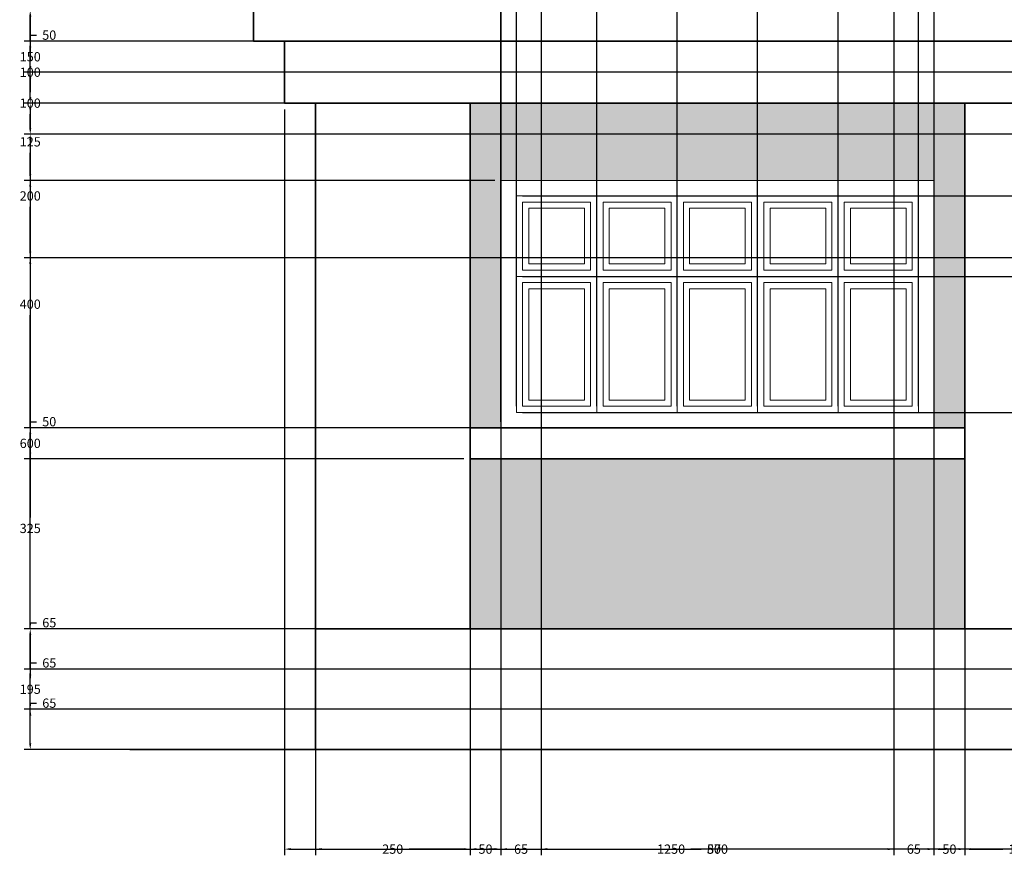
# Model space of a CAD drawing. Units: millimetres. Extents: x 937 to 4561, y 2711 to 5748.
# Tile 1 of 8: x 951 to 2543, y 2711 to 4062. Entities that reach past the tile are written whole.
import ezdxf

# ---------------------------------------------------------------- set-up
doc = ezdxf.new("R2010")
doc.units = ezdxf.units.MM
doc.header["$MEASUREMENT"] = 0
for name, color, linetype, lineweight in [('A-ANNO-DIMS', 2, 'Continuous', 18), ('A-ELEV', 7, 'Continuous', 35), ('A-GLAZ', 4, 'Continuous', 18), ('A-WALL-PATT', 8, 'Continuous', 13)]:
    doc.layers.add(name, color=color, linetype=linetype, lineweight=lineweight)
doc.styles.get("Standard").update_dxf_attribs({"font": 'arial.ttf'})
doc.dimstyles.get("Standard").update_dxf_attribs({"dimtxt": 15, "dimasz": 10, "dimexe": 10, "dimexo": 10, "dimgap": 10, "dimtad": 0, "dimtih": 1, "dimtoh": 1, "dimdec": 0, "dimzin": 0, "dimdsep": 46, "dimtxsty": 'Standard', "dimcen": 5, "dimadec": 0, "dimazin": 0, "dimtfac": 1, "dimtdec": 0, "dimtofl": 0, "dimtmove": 0, "dimatfit": 3, "dimfxl": 1, "dimtolj": 1, "dimtzin": 0, "dimarcsym": 0})

# ---------------------------------------------------------------- blocks, each defined once
blk = doc.blocks.new('*D4')
at = {"layer": 'A-ANNO-DIMS', "color": 0, "lineweight": -2, "transparency": 16777216}
for p, q in [((1429.5, 3066.9), (1429.5, 2710.9)), ((1679.5, 3066.9), (1679.5, 2710.9)), ((1439.5, 2720.9), (1527.8, 2720.9)), ((1669.5, 2720.9), (1581.2, 2720.9))]:
    blk.add_line(p, q, dxfattribs=at)
at = {"layer": 'A-ANNO-DIMS', "color": 0, "transparency": 16777216}
for points in [[(1439.5, 2722.6), (1439.5, 2719.2), (1429.5, 2720.9)], [(1669.5, 2722.6), (1669.5, 2719.2), (1679.5, 2720.9)]]:
    blk.add_solid(points, dxfattribs=at)
at = {"layer": 'Defpoints', "color": 0, "transparency": 16777216}
for p in [(1429.5, 3076.9), (1679.5, 3076.9), (1679.5, 2720.9)]:
    blk.add_point(p, dxfattribs=at)
at = {"layer": 'A-ANNO-DIMS', "color": 0, "transparency": 16777216, "insert": (1554.5, 2720.9), "char_height": 15, "attachment_point": 5}
blk.add_mtext('\\A1;250', dxfattribs=at)
blk = doc.blocks.new('*D5')
at = {"layer": 'A-ANNO-DIMS', "color": 0, "lineweight": -2, "transparency": 16777216}
for p, q in [((1679.5, 3066.9), (1679.5, 2710.9)), ((2479.5, 3066.9), (2479.5, 2710.9)), ((1689.5, 2720.9), (2052.9, 2720.9)), ((2469.5, 2720.9), (2106, 2720.9))]:
    blk.add_line(p, q, dxfattribs=at)
at = {"layer": 'A-ANNO-DIMS', "color": 0, "transparency": 16777216}
for points in [[(1689.5, 2722.6), (1689.5, 2719.2), (1679.5, 2720.9)], [(2469.5, 2722.6), (2469.5, 2719.2), (2479.5, 2720.9)]]:
    blk.add_solid(points, dxfattribs=at)
at = {"layer": 'Defpoints', "color": 0, "transparency": 16777216}
for p in [(1679.5, 3076.9), (2479.5, 3076.9), (2479.5, 2720.9)]:
    blk.add_point(p, dxfattribs=at)
at = {"layer": 'A-ANNO-DIMS', "color": 0, "transparency": 16777216, "insert": (2079.5, 2720.9), "char_height": 15, "attachment_point": 5}
blk.add_mtext('\\A1;800', dxfattribs=at)
blk = doc.blocks.new('*D6')
at = {"layer": 'A-ANNO-DIMS', "color": 0, "lineweight": -2, "transparency": 16777216}
for p, q in [((2479.5, 3066.9), (2479.5, 2710.9)), ((2654.5, 3066.9), (2654.5, 2710.9)), ((2489.5, 2720.9), (2541.1, 2720.9)), ((2644.5, 2720.9), (2592.9, 2720.9))]:
    blk.add_line(p, q, dxfattribs=at)
at = {"layer": 'A-ANNO-DIMS', "color": 0, "transparency": 16777216}
for points in [[(2489.5, 2722.6), (2489.5, 2719.2), (2479.5, 2720.9)], [(2644.5, 2722.6), (2644.5, 2719.2), (2654.5, 2720.9)]]:
    blk.add_solid(points, dxfattribs=at)
at = {"layer": 'Defpoints', "color": 0, "transparency": 16777216}
for p in [(2479.5, 3076.9), (2654.5, 3076.9), (2654.5, 2720.9)]:
    blk.add_point(p, dxfattribs=at)
at = {"layer": 'A-ANNO-DIMS', "color": 0, "transparency": 16777216, "insert": (2567, 2720.9), "char_height": 15, "attachment_point": 5}
blk.add_mtext('\\A1;175', dxfattribs=at)
blk = doc.blocks.new('*D27')
at = {"layer": 'A-ANNO-DIMS', "color": 0, "lineweight": -2, "transparency": 16777216}
for p, q in [((1729.5, 4391.9), (1729.5, 2710.9)), ((1794.5, 4391.9), (1794.5, 2710.9)), ((1719.5, 2720.9), (1709.5, 2720.9)), ((1804.5, 2720.9), (1814.5, 2720.9))]:
    blk.add_line(p, q, dxfattribs=at)
at = {"layer": 'A-ANNO-DIMS', "color": 0, "transparency": 16777216}
for points in [[(1719.5, 2722.6), (1719.5, 2719.2), (1729.5, 2720.9)], [(1804.5, 2722.6), (1804.5, 2719.2), (1794.5, 2720.9)]]:
    blk.add_solid(points, dxfattribs=at)
at = {"layer": 'Defpoints', "color": 0, "transparency": 16777216}
for p in [(1729.5, 4401.9), (1794.5, 4401.9), (1794.5, 2720.9)]:
    blk.add_point(p, dxfattribs=at)
at = {"layer": 'A-ANNO-DIMS', "color": 0, "transparency": 16777216, "insert": (1762, 2720.9), "char_height": 15, "attachment_point": 5}
blk.add_mtext('\\A1;65', dxfattribs=at)
blk = doc.blocks.new('*D28')
at = {"layer": 'A-ANNO-DIMS', "color": 0, "lineweight": -2, "transparency": 16777216}
for p, q in [((1794.5, 4391.9), (1794.5, 2710.9)), ((2364.5, 4391.9), (2364.5, 2710.9)), ((1804.5, 2720.9), (2052.9, 2720.9)), ((2354.5, 2720.9), (2106, 2720.9))]:
    blk.add_line(p, q, dxfattribs=at)
at = {"layer": 'A-ANNO-DIMS', "color": 0, "transparency": 16777216}
for points in [[(1804.5, 2722.6), (1804.5, 2719.2), (1794.5, 2720.9)], [(2354.5, 2722.6), (2354.5, 2719.2), (2364.5, 2720.9)]]:
    blk.add_solid(points, dxfattribs=at)
at = {"layer": 'Defpoints', "color": 0, "transparency": 16777216}
for p in [(1794.5, 4401.9), (2364.5, 4401.9), (2364.5, 2720.9)]:
    blk.add_point(p, dxfattribs=at)
at = {"layer": 'A-ANNO-DIMS', "color": 0, "transparency": 16777216, "insert": (2079.5, 2720.9), "char_height": 15, "attachment_point": 5}
blk.add_mtext('\\A1;570', dxfattribs=at)
blk = doc.blocks.new('*D29')
at = {"layer": 'A-ANNO-DIMS', "color": 0, "lineweight": -2, "transparency": 16777216}
for p, q in [((2364.5, 4391.9), (2364.5, 2710.9)), ((2429.5, 4391.9), (2429.5, 2710.9)), ((2354.5, 2720.9), (2344.5, 2720.9)), ((2439.5, 2720.9), (2449.5, 2720.9))]:
    blk.add_line(p, q, dxfattribs=at)
at = {"layer": 'A-ANNO-DIMS', "color": 0, "transparency": 16777216}
for points in [[(2354.5, 2722.6), (2354.5, 2719.2), (2364.5, 2720.9)], [(2439.5, 2722.6), (2439.5, 2719.2), (2429.5, 2720.9)]]:
    blk.add_solid(points, dxfattribs=at)
at = {"layer": 'Defpoints', "color": 0, "transparency": 16777216}
for p in [(2364.5, 4401.9), (2429.5, 4401.9), (2429.5, 2720.9)]:
    blk.add_point(p, dxfattribs=at)
at = {"layer": 'A-ANNO-DIMS', "color": 0, "transparency": 16777216, "insert": (2397, 2720.9), "char_height": 15, "attachment_point": 5}
blk.add_mtext('\\A1;65', dxfattribs=at)
blk = doc.blocks.new('*D35')
at = {"layer": 'A-ANNO-DIMS', "color": 0, "lineweight": -2, "transparency": 16777216}
for p, q in [((1679.5, 3391.9), (1679.5, 2710.9)), ((1729.5, 3391.9), (1729.5, 2710.9)), ((1669.5, 2720.9), (1659.5, 2720.9)), ((1739.5, 2720.9), (1749.5, 2720.9))]:
    blk.add_line(p, q, dxfattribs=at)
at = {"layer": 'A-ANNO-DIMS', "color": 0, "transparency": 16777216}
for points in [[(1669.5, 2722.6), (1669.5, 2719.2), (1679.5, 2720.9)], [(1739.5, 2722.6), (1739.5, 2719.2), (1729.5, 2720.9)]]:
    blk.add_solid(points, dxfattribs=at)
at = {"layer": 'Defpoints', "color": 0, "transparency": 16777216}
for p in [(1679.5, 3401.9), (1729.5, 3401.9), (1729.5, 2720.9)]:
    blk.add_point(p, dxfattribs=at)
at = {"layer": 'A-ANNO-DIMS', "color": 0, "transparency": 16777216, "insert": (1704.5, 2720.9), "char_height": 15, "attachment_point": 5}
blk.add_mtext('\\A1;50', dxfattribs=at)
blk = doc.blocks.new('*D36')
at = {"layer": 'A-ANNO-DIMS', "color": 0, "lineweight": -2, "transparency": 16777216}
for p, q in [((2429.5, 3391.9), (2429.5, 2710.9)), ((2479.5, 3391.9), (2479.5, 2710.9)), ((2419.5, 2720.9), (2409.5, 2720.9)), ((2489.5, 2720.9), (2499.5, 2720.9))]:
    blk.add_line(p, q, dxfattribs=at)
at = {"layer": 'A-ANNO-DIMS', "color": 0, "transparency": 16777216}
for points in [[(2419.5, 2722.6), (2419.5, 2719.2), (2429.5, 2720.9)], [(2489.5, 2722.6), (2489.5, 2719.2), (2479.5, 2720.9)]]:
    blk.add_solid(points, dxfattribs=at)
at = {"layer": 'Defpoints', "color": 0, "transparency": 16777216}
for p in [(2429.5, 3401.9), (2479.5, 3401.9), (2479.5, 2720.9)]:
    blk.add_point(p, dxfattribs=at)
at = {"layer": 'A-ANNO-DIMS', "color": 0, "transparency": 16777216, "insert": (2454.5, 2720.9), "char_height": 15, "attachment_point": 5}
blk.add_mtext('\\A1;50', dxfattribs=at)
blk = doc.blocks.new('*D37')
at = {"layer": 'A-ANNO-DIMS', "color": 0, "lineweight": -2, "transparency": 16777216}
for p, q in [((1729.5, 3411.9), (1729.5, 5747.9)), ((1754.5, 3436.9), (1754.5, 5747.9)), ((1719.5, 5737.9), (1709.5, 5737.9)), ((1764.5, 5737.9), (1774.5, 5737.9))]:
    blk.add_line(p, q, dxfattribs=at)
at = {"layer": 'A-ANNO-DIMS', "color": 0, "transparency": 16777216}
for points in [[(1719.5, 5739.6), (1719.5, 5736.2), (1729.5, 5737.9)], [(1764.5, 5739.6), (1764.5, 5736.2), (1754.5, 5737.9)]]:
    blk.add_solid(points, dxfattribs=at)
at = {"layer": 'Defpoints', "color": 0, "transparency": 16777216}
for p in [(1754.5, 5737.9), (1754.5, 3426.9), (1729.5, 3401.9)]:
    blk.add_point(p, dxfattribs=at)
at = {"layer": 'A-ANNO-DIMS', "color": 0, "transparency": 16777216, "insert": (1795.4, 5737.9), "char_height": 15, "attachment_point": 5}
blk.add_mtext('\\A1;25', dxfattribs=at)
blk = doc.blocks.new('*D38')
at = {"layer": 'A-ANNO-DIMS', "color": 0, "lineweight": -2, "transparency": 16777216}
for p, q in [((1754.5, 3436.9), (1754.5, 5747.9)), ((1884.5, 3436.9), (1884.5, 5747.9)), ((1764.5, 5737.9), (1793.6, 5737.9)), ((1874.5, 5737.9), (1845.3, 5737.9))]:
    blk.add_line(p, q, dxfattribs=at)
at = {"layer": 'A-ANNO-DIMS', "color": 0, "transparency": 16777216}
for points in [[(1764.5, 5739.6), (1764.5, 5736.2), (1754.5, 5737.9)], [(1874.5, 5739.6), (1874.5, 5736.2), (1884.5, 5737.9)]]:
    blk.add_solid(points, dxfattribs=at)
at = {"layer": 'Defpoints', "color": 0, "transparency": 16777216}
for p in [(1884.5, 5737.9), (1754.5, 3426.9), (1884.5, 3426.9)]:
    blk.add_point(p, dxfattribs=at)
at = {"layer": 'A-ANNO-DIMS', "color": 0, "transparency": 16777216, "insert": (1819.5, 5737.9), "char_height": 15, "attachment_point": 5}
blk.add_mtext('\\A1;130', dxfattribs=at)
blk = doc.blocks.new('*D39')
at = {"layer": 'A-ANNO-DIMS', "color": 0, "lineweight": -2, "transparency": 16777216}
for p, q in [((1884.5, 3436.9), (1884.5, 5747.9)), ((2014.5, 3436.9), (2014.5, 5747.9)), ((1894.5, 5737.9), (1923.6, 5737.9)), ((2004.5, 5737.9), (1975.3, 5737.9))]:
    blk.add_line(p, q, dxfattribs=at)
at = {"layer": 'A-ANNO-DIMS', "color": 0, "transparency": 16777216}
for points in [[(1894.5, 5739.6), (1894.5, 5736.2), (1884.5, 5737.9)], [(2004.5, 5739.6), (2004.5, 5736.2), (2014.5, 5737.9)]]:
    blk.add_solid(points, dxfattribs=at)
at = {"layer": 'Defpoints', "color": 0, "transparency": 16777216}
for p in [(2014.5, 5737.9), (1884.5, 3426.9), (2014.5, 3426.9)]:
    blk.add_point(p, dxfattribs=at)
at = {"layer": 'A-ANNO-DIMS', "color": 0, "transparency": 16777216, "insert": (1949.5, 5737.9), "char_height": 15, "attachment_point": 5}
blk.add_mtext('\\A1;130', dxfattribs=at)
blk = doc.blocks.new('*D40')
at = {"layer": 'A-ANNO-DIMS', "color": 0, "lineweight": -2, "transparency": 16777216}
for p, q in [((2014.5, 3436.9), (2014.5, 5747.9)), ((2144.5, 3436.9), (2144.5, 5747.9)), ((2024.5, 5737.9), (2053.6, 5737.9)), ((2134.5, 5737.9), (2105.3, 5737.9))]:
    blk.add_line(p, q, dxfattribs=at)
at = {"layer": 'A-ANNO-DIMS', "color": 0, "transparency": 16777216}
for points in [[(2024.5, 5739.6), (2024.5, 5736.2), (2014.5, 5737.9)], [(2134.5, 5739.6), (2134.5, 5736.2), (2144.5, 5737.9)]]:
    blk.add_solid(points, dxfattribs=at)
at = {"layer": 'Defpoints', "color": 0, "transparency": 16777216}
for p in [(2144.5, 5737.9), (2014.5, 3426.9), (2144.5, 3426.9)]:
    blk.add_point(p, dxfattribs=at)
at = {"layer": 'A-ANNO-DIMS', "color": 0, "transparency": 16777216, "insert": (2079.5, 5737.9), "char_height": 15, "attachment_point": 5}
blk.add_mtext('\\A1;130', dxfattribs=at)
blk = doc.blocks.new('*D41')
at = {"layer": 'A-ANNO-DIMS', "color": 0, "lineweight": -2, "transparency": 16777216}
for p, q in [((2144.5, 3436.9), (2144.5, 5747.9)), ((2274.5, 3436.9), (2274.5, 5747.9)), ((2154.5, 5737.9), (2183.6, 5737.9)), ((2264.5, 5737.9), (2235.3, 5737.9))]:
    blk.add_line(p, q, dxfattribs=at)
at = {"layer": 'A-ANNO-DIMS', "color": 0, "transparency": 16777216}
for points in [[(2154.5, 5739.6), (2154.5, 5736.2), (2144.5, 5737.9)], [(2264.5, 5739.6), (2264.5, 5736.2), (2274.5, 5737.9)]]:
    blk.add_solid(points, dxfattribs=at)
at = {"layer": 'Defpoints', "color": 0, "transparency": 16777216}
for p in [(2274.5, 5737.9), (2144.5, 3426.9), (2274.5, 3426.9)]:
    blk.add_point(p, dxfattribs=at)
at = {"layer": 'A-ANNO-DIMS', "color": 0, "transparency": 16777216, "insert": (2209.5, 5737.9), "char_height": 15, "attachment_point": 5}
blk.add_mtext('\\A1;130', dxfattribs=at)
blk = doc.blocks.new('*D42')
at = {"layer": 'A-ANNO-DIMS', "color": 0, "lineweight": -2, "transparency": 16777216}
for p, q in [((2274.5, 3436.9), (2274.5, 5747.9)), ((2404.5, 3436.9), (2404.5, 5747.9)), ((2284.5, 5737.9), (2313.6, 5737.9)), ((2394.5, 5737.9), (2365.3, 5737.9))]:
    blk.add_line(p, q, dxfattribs=at)
at = {"layer": 'A-ANNO-DIMS', "color": 0, "transparency": 16777216}
for points in [[(2284.5, 5739.6), (2284.5, 5736.2), (2274.5, 5737.9)], [(2394.5, 5739.6), (2394.5, 5736.2), (2404.5, 5737.9)]]:
    blk.add_solid(points, dxfattribs=at)
at = {"layer": 'Defpoints', "color": 0, "transparency": 16777216}
for p in [(2404.5, 5737.9), (2274.5, 3426.9), (2404.5, 3426.9)]:
    blk.add_point(p, dxfattribs=at)
at = {"layer": 'A-ANNO-DIMS', "color": 0, "transparency": 16777216, "insert": (2339.5, 5737.9), "char_height": 15, "attachment_point": 5}
blk.add_mtext('\\A1;130', dxfattribs=at)
blk = doc.blocks.new('*D44')
at = {"layer": 'A-ANNO-DIMS', "color": 0, "lineweight": -2, "transparency": 16777216}
for p, q in [((1379.5, 3916.9), (1379.5, 2710.9)), ((2629.5, 3916.9), (2629.5, 2710.9)), ((1389.5, 2720.9), (1972.8, 2720.9)), ((2619.5, 2720.9), (2036.2, 2720.9))]:
    blk.add_line(p, q, dxfattribs=at)
at = {"layer": 'A-ANNO-DIMS', "color": 0, "transparency": 16777216}
for points in [[(1389.5, 2722.6), (1389.5, 2719.2), (1379.5, 2720.9)], [(2619.5, 2722.6), (2619.5, 2719.2), (2629.5, 2720.9)]]:
    blk.add_solid(points, dxfattribs=at)
at = {"layer": 'Defpoints', "color": 0, "transparency": 16777216}
for p in [(1379.5, 3926.9), (2629.5, 3926.9), (2629.5, 2720.9)]:
    blk.add_point(p, dxfattribs=at)
at = {"layer": 'A-ANNO-DIMS', "color": 0, "transparency": 16777216, "insert": (2004.5, 2720.9), "char_height": 15, "attachment_point": 5}
blk.add_mtext('\\A1;1250', dxfattribs=at)
blk = doc.blocks.new('*D55')
at = {"layer": 'A-ANNO-DIMS', "color": 0, "lineweight": -2, "transparency": 16777216}
for p, q in [((1419.5, 3076.9), (958.5, 3076.9)), ((968.5, 3066.9), (968.5, 2997.1)), ((968.5, 2891.9), (968.5, 2961.7)), ((1419.5, 2881.9), (958.5, 2881.9))]:
    blk.add_line(p, q, dxfattribs=at)
at = {"layer": 'A-ANNO-DIMS', "color": 0, "transparency": 16777216}
for points in [[(966.8, 3066.9), (970.2, 3066.9), (968.5, 3076.9)], [(966.8, 2891.9), (970.2, 2891.9), (968.5, 2881.9)]]:
    blk.add_solid(points, dxfattribs=at)
at = {"layer": 'Defpoints', "color": 0, "transparency": 16777216}
for p in [(968.5, 3076.9), (1429.5, 3076.9), (1429.5, 2881.9)]:
    blk.add_point(p, dxfattribs=at)
at = {"layer": 'A-ANNO-DIMS', "color": 0, "transparency": 16777216, "insert": (968.5, 2979.4), "char_height": 15, "attachment_point": 5}
blk.add_mtext('\\A1;195', dxfattribs=at)
blk = doc.blocks.new('*D56')
at = {"layer": 'A-ANNO-DIMS', "color": 0, "lineweight": -2, "transparency": 16777216}
for p, q in [((1719.5, 3401.9), (958.5, 3401.9)), ((968.5, 3391.9), (968.5, 3257.1)), ((968.5, 3086.9), (968.5, 3221.7)), ((1419.5, 3076.9), (958.5, 3076.9))]:
    blk.add_line(p, q, dxfattribs=at)
at = {"layer": 'A-ANNO-DIMS', "color": 0, "transparency": 16777216}
for points in [[(966.8, 3391.9), (970.2, 3391.9), (968.5, 3401.9)], [(966.8, 3086.9), (970.2, 3086.9), (968.5, 3076.9)]]:
    blk.add_solid(points, dxfattribs=at)
at = {"layer": 'Defpoints', "color": 0, "transparency": 16777216}
for p in [(968.5, 3401.9), (1729.5, 3401.9), (1429.5, 3076.9)]:
    blk.add_point(p, dxfattribs=at)
at = {"layer": 'A-ANNO-DIMS', "color": 0, "transparency": 16777216, "insert": (968.5, 3239.4), "char_height": 15, "attachment_point": 5}
blk.add_mtext('\\A1;325', dxfattribs=at)
blk = doc.blocks.new('*D57')
at = {"layer": 'A-ANNO-DIMS', "color": 0, "lineweight": -2, "transparency": 16777216}
for p, q in [((1719.5, 3801.9), (958.5, 3801.9)), ((968.5, 3791.9), (968.5, 3619.6)), ((968.5, 3411.9), (968.5, 3584.2)), ((1719.5, 3401.9), (958.5, 3401.9))]:
    blk.add_line(p, q, dxfattribs=at)
at = {"layer": 'A-ANNO-DIMS', "color": 0, "transparency": 16777216}
for points in [[(966.8, 3791.9), (970.2, 3791.9), (968.5, 3801.9)], [(966.8, 3411.9), (970.2, 3411.9), (968.5, 3401.9)]]:
    blk.add_solid(points, dxfattribs=at)
at = {"layer": 'Defpoints', "color": 0, "transparency": 16777216}
for p in [(968.5, 3801.9), (1729.5, 3801.9), (1729.5, 3401.9)]:
    blk.add_point(p, dxfattribs=at)
at = {"layer": 'A-ANNO-DIMS', "color": 0, "transparency": 16777216, "insert": (968.5, 3601.9), "char_height": 15, "attachment_point": 5}
blk.add_mtext('\\A1;400', dxfattribs=at)
blk = doc.blocks.new('*D58')
at = {"layer": 'A-ANNO-DIMS', "color": 0, "lineweight": -2, "transparency": 16777216}
for p, q in [((1419.5, 3926.9), (958.5, 3926.9)), ((968.5, 3916.9), (968.5, 3882.1)), ((968.5, 3811.9), (968.5, 3846.7)), ((1719.5, 3801.9), (958.5, 3801.9))]:
    blk.add_line(p, q, dxfattribs=at)
at = {"layer": 'A-ANNO-DIMS', "color": 0, "transparency": 16777216}
for points in [[(966.8, 3916.9), (970.2, 3916.9), (968.5, 3926.9)], [(966.8, 3811.9), (970.2, 3811.9), (968.5, 3801.9)]]:
    blk.add_solid(points, dxfattribs=at)
at = {"layer": 'Defpoints', "color": 0, "transparency": 16777216}
for p in [(968.5, 3926.9), (1429.5, 3926.9), (1729.5, 3801.9)]:
    blk.add_point(p, dxfattribs=at)
at = {"layer": 'A-ANNO-DIMS', "color": 0, "transparency": 16777216, "insert": (968.5, 3864.4), "char_height": 15, "attachment_point": 5}
blk.add_mtext('\\A1;125', dxfattribs=at)
blk = doc.blocks.new('*D59')
at = {"layer": 'A-ANNO-DIMS', "color": 0, "lineweight": -2, "transparency": 16777216}
for p, q in [((1419.5, 4076.9), (958.5, 4076.9)), ((968.5, 4066.9), (968.5, 4019.6)), ((968.5, 3936.9), (968.5, 3984.2)), ((1419.5, 3926.9), (958.5, 3926.9))]:
    blk.add_line(p, q, dxfattribs=at)
at = {"layer": 'A-ANNO-DIMS', "color": 0, "transparency": 16777216}
for points in [[(966.8, 4066.9), (970.2, 4066.9), (968.5, 4076.9)], [(966.8, 3936.9), (970.2, 3936.9), (968.5, 3926.9)]]:
    blk.add_solid(points, dxfattribs=at)
at = {"layer": 'Defpoints', "color": 0, "transparency": 16777216}
for p in [(968.5, 4076.9), (1429.5, 4076.9), (1429.5, 3926.9)]:
    blk.add_point(p, dxfattribs=at)
at = {"layer": 'A-ANNO-DIMS', "color": 0, "transparency": 16777216, "insert": (968.5, 4001.9), "char_height": 15, "attachment_point": 5}
blk.add_mtext('\\A1;150', dxfattribs=at)
blk = doc.blocks.new('*D64')
at = {"layer": 'A-ANNO-DIMS', "color": 0, "lineweight": -2, "transparency": 16777216}
for p, q in [((1319.5, 4076.9), (958.5, 4076.9)), ((968.5, 4076.9), (968.5, 4086.9)), ((968.5, 4086.9), (978.5, 4086.9)), ((968.5, 4036.9), (968.5, 4066.9)), ((1319.5, 4026.9), (958.5, 4026.9))]:
    blk.add_line(p, q, dxfattribs=at)
at = {"layer": 'A-ANNO-DIMS', "color": 0, "transparency": 16777216}
for points in [[(966.8, 4066.9), (970.2, 4066.9), (968.5, 4076.9)], [(966.8, 4036.9), (970.2, 4036.9), (968.5, 4026.9)]]:
    blk.add_solid(points, dxfattribs=at)
at = {"layer": 'Defpoints', "color": 0, "transparency": 16777216}
for p in [(968.5, 4076.9), (1329.5, 4076.9), (1329.5, 4026.9)]:
    blk.add_point(p, dxfattribs=at)
at = {"layer": 'A-ANNO-DIMS', "color": 0, "transparency": 16777216, "insert": (999.2, 4086.9), "char_height": 15, "attachment_point": 5}
blk.add_mtext('\\A1;50', dxfattribs=at)
blk = doc.blocks.new('*D65')
at = {"layer": 'A-ANNO-DIMS', "color": 0, "lineweight": -2, "transparency": 16777216}
for p, q in [((1369.5, 4026.9), (958.5, 4026.9)), ((968.5, 4016.9), (968.5, 3994.6)), ((968.5, 3936.9), (968.5, 3959.2)), ((1369.5, 3926.9), (958.5, 3926.9))]:
    blk.add_line(p, q, dxfattribs=at)
at = {"layer": 'A-ANNO-DIMS', "color": 0, "transparency": 16777216}
for points in [[(966.8, 4016.9), (970.2, 4016.9), (968.5, 4026.9)], [(966.8, 3936.9), (970.2, 3936.9), (968.5, 3926.9)]]:
    blk.add_solid(points, dxfattribs=at)
at = {"layer": 'Defpoints', "color": 0, "transparency": 16777216}
for p in [(968.5, 4026.9), (1379.5, 4026.9), (1379.5, 3926.9)]:
    blk.add_point(p, dxfattribs=at)
at = {"layer": 'A-ANNO-DIMS', "color": 0, "transparency": 16777216, "insert": (968.5, 3976.9), "char_height": 15, "attachment_point": 5}
blk.add_mtext('\\A1;100', dxfattribs=at)
blk = doc.blocks.new('*D71')
at = {"layer": 'A-ANNO-DIMS', "color": 0, "lineweight": -2, "transparency": 16777216}
for p, q in [((968.5, 3401.9), (968.5, 3411.9)), ((968.5, 3411.9), (978.5, 3411.9)), ((1669.5, 3401.9), (958.5, 3401.9)), ((968.5, 3361.9), (968.5, 3391.9)), ((1669.5, 3351.9), (958.5, 3351.9))]:
    blk.add_line(p, q, dxfattribs=at)
at = {"layer": 'A-ANNO-DIMS', "color": 0, "transparency": 16777216}
for points in [[(966.8, 3391.9), (970.2, 3391.9), (968.5, 3401.9)], [(966.8, 3361.9), (970.2, 3361.9), (968.5, 3351.9)]]:
    blk.add_solid(points, dxfattribs=at)
at = {"layer": 'Defpoints', "color": 0, "transparency": 16777216}
for p in [(968.5, 3401.9), (1679.5, 3401.9), (1679.5, 3351.9)]:
    blk.add_point(p, dxfattribs=at)
at = {"layer": 'A-ANNO-DIMS', "color": 0, "transparency": 16777216, "insert": (999.2, 3411.9), "char_height": 15, "attachment_point": 5}
blk.add_mtext('\\A1;50', dxfattribs=at)
blk = doc.blocks.new('*D72')
at = {"layer": 'A-ANNO-DIMS', "color": 0, "lineweight": -2, "transparency": 16777216}
for p, q in [((1764.5, 3646.9), (4500.5, 3646.9)), ((4490.5, 3636.9), (4490.5, 3554.6)), ((4490.5, 3436.9), (4490.5, 3519.2)), ((1764.5, 3426.9), (4500.5, 3426.9))]:
    blk.add_line(p, q, dxfattribs=at)
at = {"layer": 'A-ANNO-DIMS', "color": 0, "transparency": 16777216}
for points in [[(4488.8, 3636.9), (4492.2, 3636.9), (4490.5, 3646.9)], [(4488.8, 3436.9), (4492.2, 3436.9), (4490.5, 3426.9)]]:
    blk.add_solid(points, dxfattribs=at)
at = {"layer": 'Defpoints', "color": 0, "transparency": 16777216}
for p in [(1754.5, 3646.9), (4490.5, 3646.9), (1754.5, 3426.9)]:
    blk.add_point(p, dxfattribs=at)
at = {"layer": 'A-ANNO-DIMS', "color": 0, "transparency": 16777216, "insert": (4490.5, 3536.9), "char_height": 15, "attachment_point": 5}
blk.add_mtext('\\A1;220', dxfattribs=at)
blk = doc.blocks.new('*D73')
at = {"layer": 'A-ANNO-DIMS', "color": 0, "lineweight": -2, "transparency": 16777216}
for p, q in [((1764.5, 3776.9), (4500.5, 3776.9)), ((4490.5, 3766.9), (4490.5, 3729.6)), ((4490.5, 3656.9), (4490.5, 3694.2)), ((1764.5, 3646.9), (4500.5, 3646.9))]:
    blk.add_line(p, q, dxfattribs=at)
at = {"layer": 'A-ANNO-DIMS', "color": 0, "transparency": 16777216}
for points in [[(4488.8, 3766.9), (4492.2, 3766.9), (4490.5, 3776.9)], [(4488.8, 3656.9), (4492.2, 3656.9), (4490.5, 3646.9)]]:
    blk.add_solid(points, dxfattribs=at)
at = {"layer": 'Defpoints', "color": 0, "transparency": 16777216}
for p in [(1754.5, 3776.9), (4490.5, 3776.9), (1754.5, 3646.9)]:
    blk.add_point(p, dxfattribs=at)
at = {"layer": 'A-ANNO-DIMS', "color": 0, "transparency": 16777216, "insert": (4490.5, 3711.9), "char_height": 15, "attachment_point": 5}
blk.add_mtext('\\A1;130', dxfattribs=at)
blk = doc.blocks.new('*D82')
at = {"layer": 'A-ANNO-DIMS', "color": 0, "lineweight": -2, "transparency": 16777216}
for p, q in [((2719.5, 3676.9), (958.5, 3676.9)), ((968.5, 3666.9), (968.5, 3394.6)), ((968.5, 3086.9), (968.5, 3359.2)), ((2719.5, 3076.9), (958.5, 3076.9))]:
    blk.add_line(p, q, dxfattribs=at)
at = {"layer": 'A-ANNO-DIMS', "color": 0, "transparency": 16777216}
for points in [[(966.8, 3666.9), (970.2, 3666.9), (968.5, 3676.9)], [(966.8, 3086.9), (970.2, 3086.9), (968.5, 3076.9)]]:
    blk.add_solid(points, dxfattribs=at)
at = {"layer": 'Defpoints', "color": 0, "transparency": 16777216}
for p in [(968.5, 3676.9), (2729.5, 3676.9), (2729.5, 3076.9)]:
    blk.add_point(p, dxfattribs=at)
at = {"layer": 'A-ANNO-DIMS', "color": 0, "transparency": 16777216, "insert": (968.5, 3376.9), "char_height": 15, "attachment_point": 5}
blk.add_mtext('\\A1;600', dxfattribs=at)
blk = doc.blocks.new('*D83')
at = {"layer": 'A-ANNO-DIMS', "color": 0, "lineweight": -2, "transparency": 16777216}
for p, q in [((2619.5, 3876.9), (958.5, 3876.9)), ((968.5, 3866.9), (968.5, 3794.6)), ((968.5, 3686.9), (968.5, 3759.2)), ((2719.5, 3676.9), (958.5, 3676.9))]:
    blk.add_line(p, q, dxfattribs=at)
at = {"layer": 'A-ANNO-DIMS', "color": 0, "transparency": 16777216}
for points in [[(966.8, 3866.9), (970.2, 3866.9), (968.5, 3876.9)], [(966.8, 3686.9), (970.2, 3686.9), (968.5, 3676.9)]]:
    blk.add_solid(points, dxfattribs=at)
at = {"layer": 'Defpoints', "color": 0, "transparency": 16777216}
for p in [(968.5, 3876.9), (2629.5, 3876.9), (2729.5, 3676.9)]:
    blk.add_point(p, dxfattribs=at)
at = {"layer": 'A-ANNO-DIMS', "color": 0, "transparency": 16777216, "insert": (968.5, 3776.9), "char_height": 15, "attachment_point": 5}
blk.add_mtext('\\A1;200', dxfattribs=at)
blk = doc.blocks.new('*D84')
at = {"layer": 'A-ANNO-DIMS', "color": 0, "lineweight": -2, "transparency": 16777216}
for p, q in [((2569.5, 3976.9), (958.5, 3976.9)), ((968.5, 3966.9), (968.5, 3944.6)), ((968.5, 3886.9), (968.5, 3909.2)), ((2619.5, 3876.9), (958.5, 3876.9))]:
    blk.add_line(p, q, dxfattribs=at)
at = {"layer": 'A-ANNO-DIMS', "color": 0, "transparency": 16777216}
for points in [[(966.8, 3966.9), (970.2, 3966.9), (968.5, 3976.9)], [(966.8, 3886.9), (970.2, 3886.9), (968.5, 3876.9)]]:
    blk.add_solid(points, dxfattribs=at)
at = {"layer": 'Defpoints', "color": 0, "transparency": 16777216}
for p in [(968.5, 3976.9), (2579.5, 3976.9), (2629.5, 3876.9)]:
    blk.add_point(p, dxfattribs=at)
at = {"layer": 'A-ANNO-DIMS', "color": 0, "transparency": 16777216, "insert": (968.5, 3926.9), "char_height": 15, "attachment_point": 5}
blk.add_mtext('\\A1;100', dxfattribs=at)
blk = doc.blocks.new('*D85')
at = {"layer": 'A-ANNO-DIMS', "color": 0, "lineweight": -2, "transparency": 16777216}
for p, q in [((968.5, 4026.9), (968.5, 4036.9)), ((968.5, 4036.9), (978.5, 4036.9)), ((2569.5, 4026.9), (958.5, 4026.9)), ((968.5, 3986.9), (968.5, 4016.9)), ((2569.5, 3976.9), (958.5, 3976.9))]:
    blk.add_line(p, q, dxfattribs=at)
at = {"layer": 'A-ANNO-DIMS', "color": 0, "transparency": 16777216}
for points in [[(966.8, 4016.9), (970.2, 4016.9), (968.5, 4026.9)], [(966.8, 3986.9), (970.2, 3986.9), (968.5, 3976.9)]]:
    blk.add_solid(points, dxfattribs=at)
at = {"layer": 'Defpoints', "color": 0, "transparency": 16777216}
for p in [(968.5, 4026.9), (2579.5, 4026.9), (2579.5, 3976.9)]:
    blk.add_point(p, dxfattribs=at)
at = {"layer": 'A-ANNO-DIMS', "color": 0, "transparency": 16777216, "insert": (999.2, 4036.9), "char_height": 15, "attachment_point": 5}
blk.add_mtext('\\A1;50', dxfattribs=at)
blk = doc.blocks.new('*D86')
at = {"layer": 'A-ANNO-DIMS', "color": 0, "lineweight": -2, "transparency": 16777216}
for p, q in [((2569.5, 4076.9), (958.5, 4076.9)), ((968.5, 4076.9), (968.5, 4086.9)), ((968.5, 4086.9), (978.5, 4086.9)), ((968.5, 4036.9), (968.5, 4066.9)), ((2569.5, 4026.9), (958.5, 4026.9))]:
    blk.add_line(p, q, dxfattribs=at)
at = {"layer": 'A-ANNO-DIMS', "color": 0, "transparency": 16777216}
for points in [[(966.8, 4066.9), (970.2, 4066.9), (968.5, 4076.9)], [(966.8, 4036.9), (970.2, 4036.9), (968.5, 4026.9)]]:
    blk.add_solid(points, dxfattribs=at)
at = {"layer": 'Defpoints', "color": 0, "transparency": 16777216}
for p in [(968.5, 4076.9), (2579.5, 4076.9), (2579.5, 4026.9)]:
    blk.add_point(p, dxfattribs=at)
at = {"layer": 'A-ANNO-DIMS', "color": 0, "transparency": 16777216, "insert": (999.2, 4086.9), "char_height": 15, "attachment_point": 5}
blk.add_mtext('\\A1;50', dxfattribs=at)
blk = doc.blocks.new('*D99')
at = {"layer": 'A-ANNO-DIMS', "color": 0, "lineweight": -2, "transparency": 16777216}
for p, q in [((2719.5, 2946.9), (958.5, 2946.9)), ((968.5, 2946.9), (968.5, 2956.9)), ((968.5, 2956.9), (978.5, 2956.9)), ((968.5, 2891.9), (968.5, 2936.9)), ((2644.5, 2881.9), (958.5, 2881.9))]:
    blk.add_line(p, q, dxfattribs=at)
at = {"layer": 'A-ANNO-DIMS', "color": 0, "transparency": 16777216}
for points in [[(966.8, 2936.9), (970.2, 2936.9), (968.5, 2946.9)], [(966.8, 2891.9), (970.2, 2891.9), (968.5, 2881.9)]]:
    blk.add_solid(points, dxfattribs=at)
at = {"layer": 'Defpoints', "color": 0, "transparency": 16777216}
for p in [(968.5, 2946.9), (2729.5, 2946.9), (2654.5, 2881.9)]:
    blk.add_point(p, dxfattribs=at)
at = {"layer": 'A-ANNO-DIMS', "color": 0, "transparency": 16777216, "insert": (999.3, 2956.9), "char_height": 15, "attachment_point": 5}
blk.add_mtext('\\A1;65', dxfattribs=at)
blk = doc.blocks.new('*D100')
at = {"layer": 'A-ANNO-DIMS', "color": 0, "lineweight": -2, "transparency": 16777216}
for p, q in [((2719.5, 3011.9), (958.5, 3011.9)), ((968.5, 3011.9), (968.5, 3021.9)), ((968.5, 3021.9), (978.5, 3021.9)), ((968.5, 2956.9), (968.5, 3001.9)), ((2719.5, 2946.9), (958.5, 2946.9))]:
    blk.add_line(p, q, dxfattribs=at)
at = {"layer": 'A-ANNO-DIMS', "color": 0, "transparency": 16777216}
for points in [[(966.8, 3001.9), (970.2, 3001.9), (968.5, 3011.9)], [(966.8, 2956.9), (970.2, 2956.9), (968.5, 2946.9)]]:
    blk.add_solid(points, dxfattribs=at)
at = {"layer": 'Defpoints', "color": 0, "transparency": 16777216}
for p in [(968.5, 3011.9), (2729.5, 3011.9), (2729.5, 2946.9)]:
    blk.add_point(p, dxfattribs=at)
at = {"layer": 'A-ANNO-DIMS', "color": 0, "transparency": 16777216, "insert": (999.3, 3021.9), "char_height": 15, "attachment_point": 5}
blk.add_mtext('\\A1;65', dxfattribs=at)
blk = doc.blocks.new('*D101')
at = {"layer": 'A-ANNO-DIMS', "color": 0, "lineweight": -2, "transparency": 16777216}
for p, q in [((2644.5, 3076.9), (958.5, 3076.9)), ((968.5, 3076.9), (968.5, 3086.9)), ((968.5, 3086.9), (978.5, 3086.9)), ((968.5, 3021.9), (968.5, 3066.9)), ((2719.5, 3011.9), (958.5, 3011.9))]:
    blk.add_line(p, q, dxfattribs=at)
at = {"layer": 'A-ANNO-DIMS', "color": 0, "transparency": 16777216}
for points in [[(966.8, 3066.9), (970.2, 3066.9), (968.5, 3076.9)], [(966.8, 3021.9), (970.2, 3021.9), (968.5, 3011.9)]]:
    blk.add_solid(points, dxfattribs=at)
at = {"layer": 'Defpoints', "color": 0, "transparency": 16777216}
for p in [(968.5, 3076.9), (2654.5, 3076.9), (2729.5, 3011.9)]:
    blk.add_point(p, dxfattribs=at)
at = {"layer": 'A-ANNO-DIMS', "color": 0, "transparency": 16777216, "insert": (999.3, 3086.9), "char_height": 15, "attachment_point": 5}
blk.add_mtext('\\A1;65', dxfattribs=at)

msp = doc.modelspace()

# ---------------------------------------------------------------- hatches: boundary and pattern name
at = {"layer": 'A-WALL-PATT'}
h = msp.add_hatch(dxfattribs=at)
h.set_pattern_fill('AR-SAND', color=256, scale=15)
h.paths.add_polyline_path([(2429.4852, 4351.9013), (2364.4852, 4351.9013), (1729.4852, 4351.9013), (1729.4852, 4076.9013), (2429.4852, 4076.9013)])
h.paths.add_polyline_path([(2479.4852, 3926.9013), (1679.4852, 3926.9013), (1679.4852, 3401.9013), (1729.4852, 3401.9013), (1729.4852, 3801.9013), (2429.4852, 3801.9013), (2429.4852, 3401.9013), (2479.4852, 3401.9013)])
h.paths.add_polyline_path([(2479.4852, 3351.9013), (1679.4852, 3351.9013), (1679.4852, 3076.9013), (2479.4852, 3076.9013)])

# ---------------------------------------------------------------- linework, layer by layer
at = {"layer": 'A-ELEV'}
for p, q in [((1329.4852, 4076.9013), (1329.4852, 4026.9013)), ((1329.4852, 4026.9013), (1379.4852, 4026.9013)), ((1379.4852, 4026.9013), (1429.4852, 4026.9013)), ((1379.4852, 4026.9013), (1379.4852, 3926.9013)), ((1429.4852, 4026.9013), (3479.4852, 4026.9013)), ((1379.4852, 3926.9013), (1429.4852, 3926.9013)), ((1429.4852, 2881.9013), (1429.4852, 3926.9013)), ((1429.4852, 3926.9013), (2629.4852, 3926.9013)), ((1679.4852, 3076.9013), (1679.4852, 3926.9013)), ((2479.4852, 3076.9013), (2479.4852, 3926.9013)), ((1679.4852, 3401.9013), (2479.4852, 3401.9013)), ((1679.4852, 3351.9013), (2479.4852, 3351.9013)), ((1429.4852, 3076.9013), (4029.4852, 3076.9013)), ((1429.4852, 2881.9013), (1129.4852, 2881.9013)), ((1429.4852, 2881.9013), (4029.4852, 2881.9013))]:
    msp.add_line(p, q, dxfattribs=at)
at = {"layer": 'A-GLAZ'}
for p, q in [((1884.4852, 3776.9013), (1884.4852, 3426.9013)), ((2014.4852, 3776.9013), (2014.4852, 3426.9013)), ((2144.4852, 3776.9013), (2144.4852, 3426.9013)), ((2274.4852, 3776.9013), (2274.4852, 3426.9013)), ((2404.4852, 3776.9013), (2404.4852, 3426.9013)), ((1729.4852, 3401.9013), (1729.4852, 3726.9013)), ((1754.4852, 3646.9013), (2404.4852, 3646.9013))]:
    msp.add_line(p, q, dxfattribs=at)
for points in [[(1729.4852, 3801.9013), (2429.4852, 3801.9013), (2429.4852, 3401.9013), (1729.4852, 3401.9013)], [(1754.4852, 3776.9013), (1884.4852, 3776.9013), (1884.4852, 3646.9013), (1754.4852, 3646.9013)], [(1884.4852, 3776.9013), (2014.4852, 3776.9013), (2014.4852, 3646.9013), (1884.4852, 3646.9013)], [(2014.4852, 3776.9013), (2144.4852, 3776.9013), (2144.4852, 3646.9013), (2014.4852, 3646.9013)], [(2144.4852, 3776.9013), (2274.4852, 3776.9013), (2274.4852, 3646.9013), (2144.4852, 3646.9013)], [(2274.4852, 3776.9013), (2404.4852, 3776.9013), (2404.4852, 3646.9013), (2274.4852, 3646.9013)], [(1764.4852, 3766.9013), (1874.4852, 3766.9013), (1874.4852, 3656.9013), (1764.4852, 3656.9013)], [(1774.4852, 3756.9013), (1864.4852, 3756.9013), (1864.4852, 3666.9013), (1774.4852, 3666.9013)], [(1894.4852, 3766.9013), (2004.4852, 3766.9013), (2004.4852, 3656.9013), (1894.4852, 3656.9013)], [(1904.4852, 3756.9013), (1994.4852, 3756.9013), (1994.4852, 3666.9013), (1904.4852, 3666.9013)], [(2024.4852, 3766.9013), (2134.4852, 3766.9013), (2134.4852, 3656.9013), (2024.4852, 3656.9013)], [(2034.4852, 3756.9013), (2124.4852, 3756.9013), (2124.4852, 3666.9013), (2034.4852, 3666.9013)], [(2154.4852, 3766.9013), (2264.4852, 3766.9013), (2264.4852, 3656.9013), (2154.4852, 3656.9013)], [(2164.4852, 3756.9013), (2254.4852, 3756.9013), (2254.4852, 3666.9013), (2164.4852, 3666.9013)], [(2284.4852, 3766.9013), (2394.4852, 3766.9013), (2394.4852, 3656.9013), (2284.4852, 3656.9013)], [(2294.4852, 3756.9013), (2384.4852, 3756.9013), (2384.4852, 3666.9013), (2294.4852, 3666.9013)], [(1754.4852, 3646.9013), (1884.4852, 3646.9013), (1884.4852, 3426.9013), (1754.4852, 3426.9013)], [(1884.4852, 3646.9013), (2014.4852, 3646.9013), (2014.4852, 3426.9013), (1884.4852, 3426.9013)], [(2014.4852, 3646.9013), (2144.4852, 3646.9013), (2144.4852, 3426.9013), (2014.4852, 3426.9013)], [(2144.4852, 3646.9013), (2274.4852, 3646.9013), (2274.4852, 3426.9013), (2144.4852, 3426.9013)], [(2274.4852, 3646.9013), (2404.4852, 3646.9013), (2404.4852, 3426.9013), (2274.4852, 3426.9013)], [(1764.4852, 3636.9013), (1874.4852, 3636.9013), (1874.4852, 3436.9013), (1764.4852, 3436.9013)], [(1894.4852, 3636.9013), (2004.4852, 3636.9013), (2004.4852, 3436.9013), (1894.4852, 3436.9013)], [(2024.4852, 3636.9013), (2134.4852, 3636.9013), (2134.4852, 3436.9013), (2024.4852, 3436.9013)], [(2154.4852, 3636.9013), (2264.4852, 3636.9013), (2264.4852, 3436.9013), (2154.4852, 3436.9013)], [(2284.4852, 3636.9013), (2394.4852, 3636.9013), (2394.4852, 3436.9013), (2284.4852, 3436.9013)], [(1774.4852, 3626.9013), (1864.4852, 3626.9013), (1864.4852, 3446.9013), (1774.4852, 3446.9013)], [(1904.4852, 3626.9013), (1994.4852, 3626.9013), (1994.4852, 3446.9013), (1904.4852, 3446.9013)], [(2034.4852, 3626.9013), (2124.4852, 3626.9013), (2124.4852, 3446.9013), (2034.4852, 3446.9013)], [(2164.4852, 3626.9013), (2254.4852, 3626.9013), (2254.4852, 3446.9013), (2164.4852, 3446.9013)], [(2294.4852, 3626.9013), (2384.4852, 3626.9013), (2384.4852, 3446.9013), (2294.4852, 3446.9013)]]:
    msp.add_lwpolyline(points, close=True, dxfattribs=at)

# ---------------------------------------------------------------- dimensions: what is measured, and where the dimension line sits
at = {"layer": 'A-ANNO-DIMS'}
for base, p1, p2, picture, middle in [((1754.4852, 5737.9013), (1729.4852, 3401.9013), (1754.4852, 3426.9013), '*D37', (1795.4129, 5737.9013)), ((1884.4852, 5737.9013), (1754.4852, 3426.9013), (1884.4852, 3426.9013), '*D38', (1819.4852, 5737.9013)), ((2014.4852, 5737.9013), (1884.4852, 3426.9013), (2014.4852, 3426.9013), '*D39', (1949.4852, 5737.9013)), ((2144.4852, 5737.9013), (2014.4852, 3426.9013), (2144.4852, 3426.9013), '*D40', (2079.4852, 5737.9013)), ((2274.4852, 5737.9013), (2144.4852, 3426.9013), (2274.4852, 3426.9013), '*D41', (2209.4852, 5737.9013)), ((2404.4852, 5737.9013), (2274.4852, 3426.9013), (2404.4852, 3426.9013), '*D42', (2339.4852, 5737.9013)), ((1794.4852, 2720.9013), (1729.4852, 4401.9013), (1794.4852, 4401.9013), '*D27', (1761.9852, 2720.9013)), ((2364.4852, 2720.9013), (1794.4852, 4401.9013), (2364.4852, 4401.9013), '*D28', (2079.4852, 2720.9013)), ((2429.4852, 2720.9013), (2364.4852, 4401.9013), (2429.4852, 4401.9013), '*D29', (2396.9852, 2720.9013)), ((2629.4852, 2720.9013), (1379.4852, 3926.9013), (2629.4852, 3926.9013), '*D44', (2004.4852, 2720.9013)), ((1729.4852, 2720.9013), (1679.4852, 3401.9013), (1729.4852, 3401.9013), '*D35', (1704.4852, 2720.9013)), ((2479.4852, 2720.9013), (2429.4852, 3401.9013), (2479.4852, 3401.9013), '*D36', (2454.4852, 2720.9013)), ((1679.4852, 2720.9013), (1429.4852, 3076.9013), (1679.4852, 3076.9013), '*D4', (1554.4852, 2720.9013)), ((2479.4852, 2720.9013), (1679.4852, 3076.9013), (2479.4852, 3076.9013), '*D5', (2079.4852, 2720.9013)), ((2654.4852, 2720.9013), (2479.4852, 3076.9013), (2654.4852, 3076.9013), '*D6', (2566.9852, 2720.9013))]:
    dim = msp.add_linear_dim(base=base, p1=p1, p2=p2, dimstyle='Standard', override={"dimdec": 0, "dimlfac": 1, "dimrnd": 0, "dimzin": 0, "dimdsep": 46, "dimlunit": 2}, dxfattribs=at)
    dim.commit()
    dim.dimension.update_dxf_attribs({"geometry": picture, "text_midpoint": middle})
for base, p1, p2, picture, middle in [((968.4852, 4076.9013), (1329.4852, 4026.9013), (1329.4852, 4076.9013), '*D64', (999.2031, 4086.9013)), ((968.4852, 4076.9013), (2579.4852, 4026.9013), (2579.4852, 4076.9013), '*D86', (999.2031, 4086.9013)), ((968.4852, 4076.9013), (1429.4852, 3926.9013), (1429.4852, 4076.9013), '*D59', (968.4852, 4001.9013)), ((968.4852, 4026.9013), (2579.4852, 3976.9013), (2579.4852, 4026.9013), '*D85', (999.2031, 4036.9013)), ((968.4852, 4026.9013), (1379.4852, 3926.9013), (1379.4852, 4026.9013), '*D65', (968.4852, 3976.9013)), ((968.4852, 3976.9013), (2629.4852, 3876.9013), (2579.4852, 3976.9013), '*D84', (968.4852, 3926.9013)), ((968.4852, 3926.9013), (1729.4852, 3801.9013), (1429.4852, 3926.9013), '*D58', (968.4852, 3864.4013)), ((968.4852, 3876.9013), (2729.4852, 3676.9013), (2629.4852, 3876.9013), '*D83', (968.4852, 3776.9013)), ((968.4852, 3801.9013), (1729.4852, 3401.9013), (1729.4852, 3801.9013), '*D57', (968.4852, 3601.9013)), ((4490.4852, 3776.9013), (1754.4852, 3646.9013), (1754.4852, 3776.9013), '*D73', (4490.4852, 3711.9013)), ((968.4852, 3676.9013), (2729.4852, 3076.9013), (2729.4852, 3676.9013), '*D82', (968.4852, 3376.9013)), ((4490.4852, 3646.9013), (1754.4852, 3426.9013), (1754.4852, 3646.9013), '*D72', (4490.4852, 3536.9013)), ((968.4852, 3401.9013), (1679.4852, 3351.9013), (1679.4852, 3401.9013), '*D71', (999.2031, 3411.9013)), ((968.4852, 3401.9013), (1429.4852, 3076.9013), (1729.4852, 3401.9013), '*D56', (968.4852, 3239.4013)), ((968.4852, 3076.9013), (2729.4852, 3011.9013), (2654.4852, 3076.9013), '*D101', (999.3259, 3086.9013)), ((968.4852, 3076.9013), (1429.4852, 2881.9013), (1429.4852, 3076.9013), '*D55', (968.4852, 2979.4013)), ((968.4852, 3011.9013), (2729.4852, 2946.9013), (2729.4852, 3011.9013), '*D100', (999.3259, 3021.9013)), ((968.4852, 2946.9013), (2654.4852, 2881.9013), (2729.4852, 2946.9013), '*D99', (999.3259, 2956.9013))]:
    dim = msp.add_linear_dim(base=base, p1=p1, p2=p2, angle=90, dimstyle='Standard', override={"dimdec": 0, "dimlfac": 1, "dimrnd": 0, "dimzin": 0, "dimdsep": 46, "dimlunit": 2}, dxfattribs=at)
    dim.commit()
    dim.dimension.update_dxf_attribs({"geometry": picture, "text_midpoint": middle})

doc.saveas('drawing.dxf')
